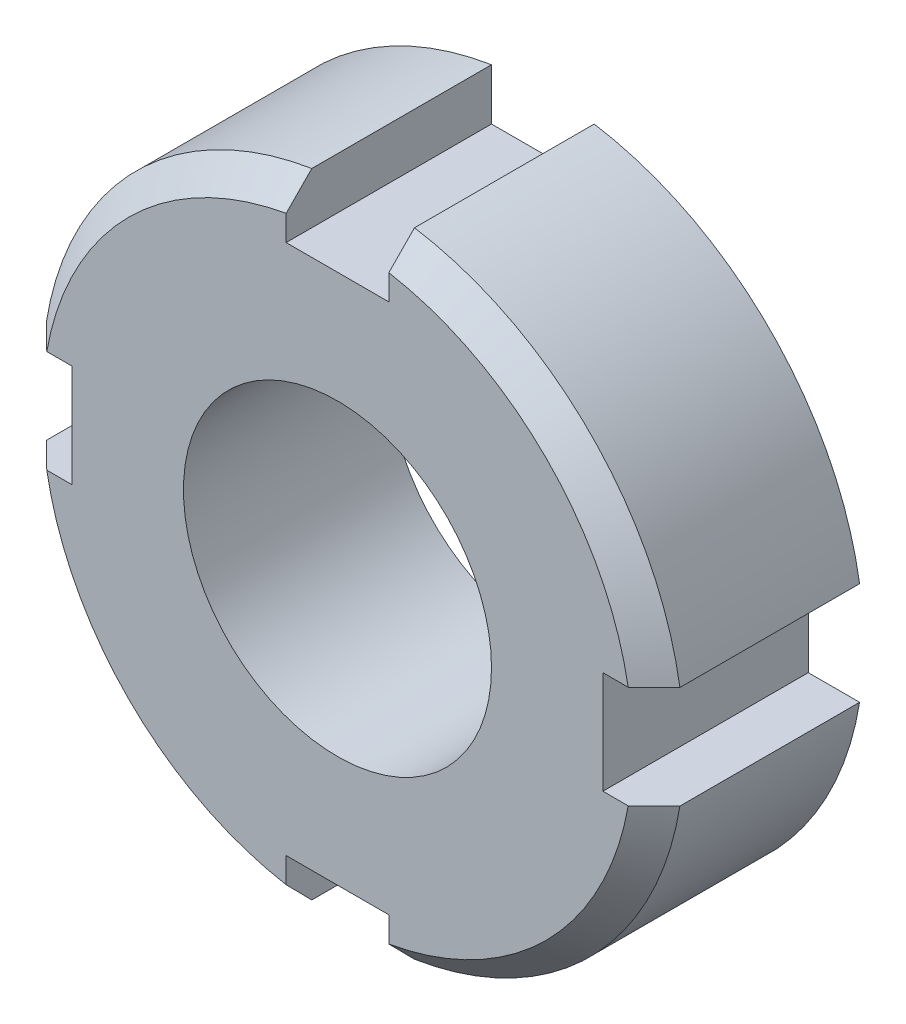
from build123d import *

# Parameters (mm, degrees)
NUT_BODY_8MM_DEPTH     = 4
M12_TAPPED_HOLE1_D     = 12
EDGE_CHAMFER_1X45_SIZE = 1


with BuildPart() as part:
    # Slotted Nut Profile → Nut Body 8mm (new, symmetric)
    with BuildSketch(Plane.XY):
        with BuildLine():
            Line((-2, 12.338962679), (-2, 10.338962679))
            Line((-2, 10.338962679), (2, 10.338962679))
            Line((2, 10.338962679), (2, 12.338962679))
            ThreePointArc((2, 12.338962679), (8.838834765, 8.838834765), (12.338962679, 2))
            Line((12.338962679, 2), (10.338962679, 2))
            Line((10.338962679, 2), (10.338962679, -2))
            Line((10.338962679, -2), (12.338962679, -2))
            ThreePointArc((12.338962679, -2), (8.838834765, -8.838834765), (2, -12.338962679))
            Line((2, -12.338962679), (2, -10.338962679))
            Line((2, -10.338962679), (-2, -10.338962679))
            Line((-2, -10.338962679), (-2, -12.338962679))
            ThreePointArc((-2, -12.338962679), (-8.838834765, -8.838834765), (-12.338962679, -2))
            Line((-12.338962679, -2), (-10.338962679, -2))
            Line((-10.338962679, -2), (-10.338962679, 2))
            Line((-10.338962679, 2), (-12.338962679, 2))
            ThreePointArc((-12.338962679, 2), (-8.838834765, 8.838834765), (-2, 12.338962679))
        make_face()
    extrude(amount=NUT_BODY_8MM_DEPTH, both=True)

    # M12 Tapped Hole1 (through all)
    with Locations(Plane.XY.offset(4)):
        with Locations((0, 0)):
            Hole(M12_TAPPED_HOLE1_D / 2)

    # Edge Chamfer 1x45°
    edge_chamfer_1x45_edges = [part.edges().sort_by_distance(p)[0] for p in [
        (-8.838834765, 8.838834765, 4),
        (-8.838834765, -8.838834765, 4),
        (8.838834765, -8.838834765, 4),
        (8.838834765, 8.838834765, 4),
    ]]
    chamfer(edge_chamfer_1x45_edges, length=EDGE_CHAMFER_1X45_SIZE)


solid = part.part
